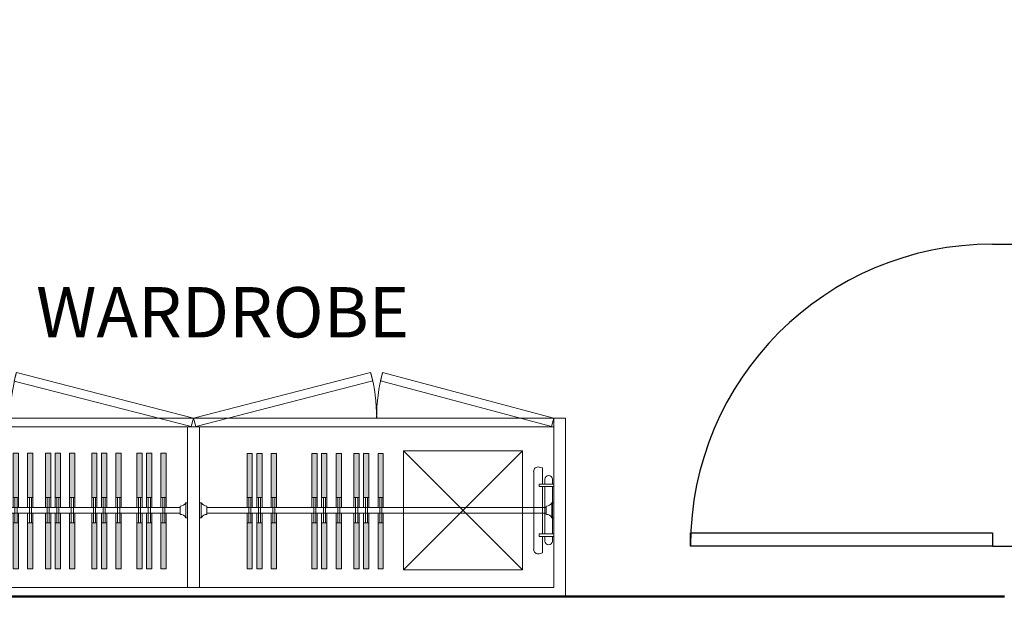
# Model space of a CAD drawing. Units: inches. Extents: x -466983 to 1020, y 324 to 318697.
# Tile 43 of 97: x 491 to 609, y 827 to 898. Entities that reach past the tile are written whole.
import ezdxf

# ---------------------------------------------------------------- set-up
doc = ezdxf.new("R2010")
doc.units = ezdxf.units.IN
doc.header["$MEASUREMENT"] = 0
for name, color, linetype, lineweight in [('A-ANNO-TEXT', 7, 'Continuous', 18), ('A-DOOR', 3, 'Continuous', 25), ('A-FLOR-PATT', 252, 'Continuous', 13), ('A-FURN', 8, 'Continuous', 18), ('A-WALL', 7, 'Continuous', 50)]:
    doc.layers.add(name, color=color, linetype=linetype, lineweight=lineweight)
doc.styles.get("Standard").update_dxf_attribs({"font": 'arial.ttf'})

# ---------------------------------------------------------------- blocks, each defined once
blk = doc.blocks.new('*U33')
for p, q in [((0, 0), (0, -6)), ((40, 0), (40, -6))]:
    blk.add_line(p, q)
blk.add_lwpolyline([(0, 0), (0, 40), (1.75, 40), (1.75, 0)], close=True)
blk.add_arc((0, 0), 40, 0, 90)
blk = doc.blocks.new('Wardrobe')
h = blk.add_hatch(color=256)
h.dxf.hatch_style = 1
h.paths.add_polyline_path([(2766.95, 1539.75), (2766.16, 1539.75), (2766.16, 1532.86), (2766.95, 1532.86)])
h.paths.add_polyline_path([(2766.95, 1529.07), (2766.16, 1529.07), (2766.16, 1522.48), (2766.95, 1522.48)])
h.paths.add_polyline_path([(2799.41, 1529.07), (2798.63, 1529.07), (2798.63, 1522.47), (2799.41, 1522.47)])
h.paths.add_polyline_path([(2799.41, 1539.75), (2798.63, 1539.75), (2798.63, 1532.86), (2799.41, 1532.86)])
h.paths.add_polyline_path([(2813.08, 1539.75), (2812.29, 1539.75), (2812.29, 1532.86), (2813.08, 1532.86)])
h.paths.add_polyline_path([(2813.08, 1529.07), (2812.29, 1529.07), (2812.29, 1522.47), (2813.08, 1522.47)])
h.paths.add_polyline_path([(2825.84, 1539.75), (2825.05, 1539.75), (2825.05, 1532.86), (2825.84, 1532.86)])
h.paths.add_polyline_path([(2825.84, 1529.07), (2825.05, 1529.07), (2825.05, 1522.47), (2825.84, 1522.47)])
h.paths.add_polyline_path([(2782.93, 1539.75), (2782.14, 1539.75), (2782.14, 1532.86), (2782.93, 1532.86)])
h.paths.add_polyline_path([(2782.93, 1529.07), (2782.14, 1529.07), (2782.14, 1522.48), (2782.93, 1522.48)])
h.paths.add_polyline_path([(2838.6, 1539.75), (2837.81, 1539.75), (2837.81, 1532.86), (2838.6, 1532.86)])
h.paths.add_polyline_path([(2838.6, 1529.07), (2837.81, 1529.07), (2837.81, 1522.47), (2838.6, 1522.47)])
h = blk.add_hatch(color=256)
h.dxf.hatch_style = 1
h.paths.add_polyline_path([(2769.11, 1539.75), (2768.32, 1539.75), (2768.32, 1532.86), (2769.11, 1532.86)])
h.paths.add_polyline_path([(2769.11, 1529.07), (2768.32, 1529.07), (2768.32, 1522.48), (2769.11, 1522.48)])
h.paths.add_polyline_path([(2801.57, 1539.75), (2800.79, 1539.75), (2800.79, 1532.86), (2801.57, 1532.86)])
h.paths.add_polyline_path([(2801.57, 1529.07), (2800.79, 1529.07), (2800.79, 1522.47), (2801.57, 1522.47)])
h.paths.add_polyline_path([(2815.24, 1539.75), (2814.45, 1539.75), (2814.45, 1532.86), (2815.24, 1532.86)])
h.paths.add_polyline_path([(2815.24, 1529.07), (2814.45, 1529.07), (2814.45, 1522.47), (2815.24, 1522.47)])
h.paths.add_polyline_path([(2828, 1529.07), (2827.21, 1529.07), (2827.21, 1522.47), (2828, 1522.47)])
h.paths.add_polyline_path([(2828, 1539.75), (2827.21, 1539.75), (2827.21, 1532.86), (2828, 1532.86)])
h.paths.add_polyline_path([(2840.76, 1539.75), (2839.97, 1539.75), (2839.97, 1532.86), (2840.76, 1532.86)])
h.paths.add_polyline_path([(2840.76, 1529.07), (2839.97, 1529.07), (2839.97, 1522.47), (2840.76, 1522.47)])
h.paths.add_polyline_path([(2785.09, 1539.75), (2784.3, 1539.75), (2784.3, 1532.86), (2785.09, 1532.86)])
h.paths.add_polyline_path([(2785.09, 1529.07), (2784.3, 1529.07), (2784.3, 1522.48), (2785.09, 1522.48)])
h = blk.add_hatch(color=256)
h.dxf.hatch_style = 1
h.paths.add_polyline_path([(2770.56, 1539.75), (2769.77, 1539.75), (2769.77, 1532.86), (2770.56, 1532.86)])
h.paths.add_polyline_path([(2770.56, 1529.07), (2769.77, 1529.07), (2769.77, 1522.48), (2770.56, 1522.48)])
h.paths.add_polyline_path([(2786.54, 1539.75), (2785.76, 1539.75), (2785.76, 1532.86), (2786.54, 1532.86)])
h.paths.add_polyline_path([(2786.54, 1529.07), (2785.76, 1529.07), (2785.76, 1522.48), (2786.54, 1522.48)])
h.paths.add_polyline_path([(2803.03, 1539.75), (2802.24, 1539.75), (2802.24, 1532.86), (2803.03, 1532.86)])
h.paths.add_polyline_path([(2803.03, 1529.07), (2802.24, 1529.07), (2802.24, 1522.47), (2803.03, 1522.47)])
h.paths.add_polyline_path([(2816.69, 1539.75), (2815.9, 1539.75), (2815.9, 1532.86), (2816.69, 1532.86)])
h.paths.add_polyline_path([(2816.69, 1529.07), (2815.9, 1529.07), (2815.9, 1522.47), (2816.69, 1522.47)])
h = blk.add_hatch(color=256)
h.dxf.hatch_style = 1
h.paths.add_polyline_path([(2773.22, 1539.75), (2772.43, 1539.75), (2772.43, 1532.86), (2773.22, 1532.86)])
h.paths.add_polyline_path([(2806.16, 1539.75), (2805.37, 1539.75), (2805.37, 1532.86), (2806.16, 1532.86)])
h.paths.add_polyline_path([(2806.16, 1529.07), (2805.37, 1529.07), (2805.37, 1522.47), (2806.16, 1522.47)])
h.paths.add_polyline_path([(2773.22, 1529.07), (2772.43, 1529.07), (2772.43, 1522.48), (2773.22, 1522.48)])
h.paths.add_polyline_path([(2819.35, 1539.75), (2818.56, 1539.75), (2818.56, 1532.86), (2819.35, 1532.86)])
h.paths.add_polyline_path([(2819.35, 1529.07), (2818.56, 1529.07), (2818.56, 1522.47), (2819.35, 1522.47)])
h.paths.add_polyline_path([(2832.33, 1539.75), (2831.54, 1539.75), (2831.54, 1532.86), (2832.33, 1532.86)])
h.paths.add_polyline_path([(2832.33, 1529.07), (2831.54, 1529.07), (2831.54, 1522.47), (2832.33, 1522.47)])
h = blk.add_hatch(color=256)
h.dxf.hatch_style = 1
h.paths.add_polyline_path([(2775.38, 1539.75), (2774.59, 1539.75), (2774.59, 1532.86), (2775.38, 1532.86)])
h.paths.add_polyline_path([(2775.38, 1529.07), (2774.59, 1529.07), (2774.59, 1522.48), (2775.38, 1522.48)])
h.paths.add_polyline_path([(2808.32, 1539.75), (2807.53, 1539.75), (2807.53, 1532.86), (2808.32, 1532.86)])
h.paths.add_polyline_path([(2808.32, 1529.07), (2807.53, 1529.07), (2807.53, 1522.47), (2808.32, 1522.47)])
h.paths.add_polyline_path([(2834.49, 1539.75), (2833.7, 1539.75), (2833.7, 1532.86), (2834.49, 1532.86)])
h.paths.add_polyline_path([(2834.49, 1529.07), (2833.7, 1529.07), (2833.7, 1522.47), (2834.49, 1522.47)])
h = blk.add_hatch(color=256)
h.dxf.hatch_style = 1
h.paths.add_polyline_path([(2776.83, 1539.75), (2776.04, 1539.75), (2776.04, 1532.86), (2776.83, 1532.86)])
h.paths.add_polyline_path([(2776.83, 1529.07), (2776.04, 1529.07), (2776.04, 1522.48), (2776.83, 1522.48)])
h.paths.add_polyline_path([(2809.77, 1539.75), (2808.98, 1539.75), (2808.98, 1532.86), (2809.77, 1532.86)])
h.paths.add_polyline_path([(2809.77, 1529.07), (2808.98, 1529.07), (2808.98, 1522.47), (2809.77, 1522.47)])
h.paths.add_polyline_path([(2821.51, 1539.75), (2820.72, 1539.75), (2820.72, 1532.86), (2821.51, 1532.86)])
h.paths.add_polyline_path([(2821.51, 1529.07), (2820.72, 1529.07), (2820.72, 1522.47), (2821.51, 1522.47)])
h = blk.add_hatch(color=256)
h.dxf.hatch_style = 1
h.paths.add_polyline_path([(2822.96, 1539.75), (2822.17, 1539.75), (2822.17, 1532.86), (2822.96, 1532.86)])
h.paths.add_polyline_path([(2822.96, 1529.07), (2822.17, 1529.07), (2822.17, 1522.47), (2822.96, 1522.47)])
h = blk.add_hatch(color=256)
h.dxf.hatch_style = 1
h.paths.add_polyline_path([(2829.45, 1539.75), (2828.67, 1539.75), (2828.67, 1532.86), (2829.45, 1532.86)])
h.paths.add_polyline_path([(2829.45, 1529.07), (2828.67, 1529.07), (2828.67, 1522.47), (2829.45, 1522.47)])
h.paths.add_polyline_path([(2842.22, 1539.75), (2841.43, 1539.75), (2841.43, 1532.86), (2842.22, 1532.86)])
h.paths.add_polyline_path([(2842.22, 1529.07), (2841.43, 1529.07), (2841.43, 1522.47), (2842.22, 1522.47)])
for p, q in [((2738.89, 1517.19, 0), (2738.89, 1543.9, 0)), ((2738.89, 1543.9, 0), (2850.18, 1543.9, 0)), ((2850.18, 1543.9, 0), (2850.18, 1517.19, 0)), ((2848.4, 1542.57, 0), (2740.67, 1542.57, 0)), ((2740.67, 1542.57, 0), (2740.67, 1517.19, 0)), ((2793.64, 1542.57, 0), (2793.64, 1518.53, 0)), ((2795.43, 1542.57, 0), (2795.43, 1518.53, 0)), ((2848.4, 1517.19, 0), (2848.4, 1542.57, 0)), ((2740.94, 1532.1, 0), (2740.67, 1532.1, 0)), ((2740.94, 1532.1, 0), (2740.67, 1532.1, 0)), ((2740.94, 1532.1, 0), (2740.94, 1529.88, 0)), ((2740.94, 1532.1, 0), (2740.94, 1529.88, 0)), ((2741.78, 1531.61, 0), (2741.78, 1530.37, 0)), ((2741.78, 1531.45, 0), (2792.53, 1531.45, 0)), ((2792.53, 1531.61, 0), (2792.53, 1530.37, 0)), ((2793.38, 1532.1, 0), (2793.38, 1529.88, 0)), ((2793.38, 1532.1, 0), (2793.38, 1529.88, 0)), ((2793.38, 1532.1, 0), (2793.64, 1532.1, 0)), ((2793.38, 1532.1, 0), (2793.64, 1532.1, 0)), ((2795.69, 1532.1, 0), (2795.43, 1532.1, 0)), ((2795.69, 1532.1, 0), (2795.43, 1532.1, 0)), ((2795.69, 1532.1, 0), (2795.69, 1529.88, 0)), ((2795.69, 1532.1, 0), (2795.69, 1529.88, 0)), ((2796.54, 1531.61, 0), (2796.54, 1530.37, 0)), ((2796.54, 1531.45, 0), (2847.29, 1531.45, 0)), ((2847.29, 1531.61, 0), (2847.29, 1530.37, 0)), ((2848.13, 1532.1, 0), (2848.13, 1529.88, 0)), ((2848.13, 1532.1, 0), (2848.13, 1529.88, 0)), ((2848.13, 1532.1, 0), (2848.4, 1532.1, 0)), ((2848.13, 1532.1, 0), (2848.4, 1532.1, 0)), ((2741.78, 1530.56, 0), (2792.53, 1530.56, 0)), ((2796.54, 1530.56, 0), (2847.29, 1530.56, 0)), ((2740.94, 1529.88, 0), (2740.67, 1529.88, 0)), ((2740.94, 1529.88, 0), (2740.67, 1529.88, 0)), ((2793.38, 1529.88, 0), (2793.64, 1529.88, 0)), ((2793.38, 1529.88, 0), (2793.64, 1529.88, 0)), ((2795.69, 1529.88, 0), (2795.43, 1529.88, 0)), ((2795.69, 1529.88, 0), (2795.43, 1529.88, 0)), ((2848.13, 1529.88, 0), (2848.4, 1529.88, 0)), ((2848.13, 1529.88, 0), (2848.4, 1529.88, 0)), ((2848.4, 1518.53, 0), (2740.67, 1518.53, 0)), ((2740.67, 1517.19, 0), (2741.02, 1518.48, 0)), ((2741.02, 1518.48, 0), (2766.6, 1511.65, 0)), ((2794.19, 1518.48, 0), (2767.71, 1511.65, 0)), ((2795.43, 1518.53, 0), (2793.64, 1518.53, 0)), ((2794.53, 1517.19, 0), (2794.19, 1518.48, 0)), ((2794.53, 1517.19, 0), (2794.88, 1518.48, 0)), ((2794.88, 1518.48, 0), (2821.36, 1511.66, 0)), ((2848.05, 1518.48, 0), (2822.47, 1511.66, 0)), ((2848.4, 1517.19, 0), (2848.05, 1518.48, 0)), ((2740.67, 1517.19, 0), (2738.89, 1517.19, 0)), ((2848.4, 1517.19, 0), (2740.67, 1517.19, 0)), ((2766.26, 1510.37, 0), (2740.67, 1517.19, 0)), ((2768.06, 1510.37, 0), (2794.53, 1517.19, 0)), ((2821.01, 1510.37, 0), (2794.53, 1517.19, 0)), ((2822.81, 1510.37, 0), (2848.4, 1517.19, 0)), ((2850.18, 1517.19, 0), (2848.4, 1517.19, 0)), ((2766.6, 1511.65, 0), (2766.26, 1510.37, 0)), ((2767.71, 1511.65, 0), (2768.06, 1510.37, 0)), ((2821.36, 1511.66, 0), (2821.01, 1510.37, 0)), ((2822.47, 1511.66, 0), (2822.81, 1510.37, 0))]:
    blk.add_line(p, q)
at = {"ltscale": 0.106667}
for p, q in [((2745.32, 1522.09, 0), (2763.13, 1539.9, 0)), ((2745.32, 1522.09, 0), (2745.32, 1539.9, 0)), ((2745.32, 1539.9, 0), (2763.13, 1539.9, 0)), ((2763.13, 1522.09, 0), (2745.32, 1539.9, 0)), ((2763.13, 1539.9, 0), (2763.13, 1522.09, 0)), ((2763.13, 1522.09, 0), (2745.32, 1522.09, 0))]:
    blk.add_line(p, q, dxfattribs=at)
at = {"ltscale": 0.037333}
for p, q in [((2766.16, 1531.37, 0), (2766.16, 1539.75, 0)), ((2766.16, 1539.75, 0), (2766.95, 1539.75, 0)), ((2766.95, 1539.75, 0), (2766.95, 1531.37, 0)), ((2768.32, 1531.37, 0), (2768.32, 1539.75, 0)), ((2768.32, 1539.75, 0), (2769.11, 1539.75, 0)), ((2769.11, 1539.75, 0), (2769.11, 1531.37, 0)), ((2769.77, 1531.37, 0), (2769.77, 1539.75, 0)), ((2769.77, 1539.75, 0), (2770.56, 1539.75, 0)), ((2770.56, 1539.75, 0), (2770.56, 1531.37, 0)), ((2772.43, 1531.37, 0), (2772.43, 1539.75, 0)), ((2772.43, 1539.75, 0), (2773.22, 1539.75, 0)), ((2773.22, 1539.75, 0), (2773.22, 1531.37, 0)), ((2774.59, 1531.37, 0), (2774.59, 1539.75, 0)), ((2774.59, 1539.75, 0), (2775.38, 1539.75, 0)), ((2775.38, 1539.75, 0), (2775.38, 1531.37, 0)), ((2776.04, 1531.37, 0), (2776.04, 1539.75, 0)), ((2776.04, 1539.75, 0), (2776.83, 1539.75, 0)), ((2776.83, 1539.75, 0), (2776.83, 1531.37, 0)), ((2782.14, 1531.37, 0), (2782.14, 1539.75, 0)), ((2782.14, 1539.75, 0), (2782.93, 1539.75, 0)), ((2782.93, 1539.75, 0), (2782.93, 1531.37, 0)), ((2784.3, 1531.37, 0), (2784.3, 1539.75, 0)), ((2784.3, 1539.75, 0), (2785.09, 1539.75, 0)), ((2785.09, 1539.75, 0), (2785.09, 1531.37, 0)), ((2785.76, 1531.37, 0), (2785.76, 1539.75, 0)), ((2785.76, 1539.75, 0), (2786.54, 1539.75, 0)), ((2786.54, 1539.75, 0), (2786.54, 1531.37, 0)), ((2798.63, 1531.36, 0), (2798.63, 1539.75, 0)), ((2798.63, 1539.75, 0), (2799.41, 1539.75, 0)), ((2799.41, 1539.75, 0), (2799.41, 1531.36, 0)), ((2800.79, 1531.36, 0), (2800.79, 1539.75, 0)), ((2800.79, 1539.75, 0), (2801.57, 1539.75, 0)), ((2801.57, 1539.75, 0), (2801.57, 1531.36, 0)), ((2802.24, 1531.36, 0), (2802.24, 1539.75, 0)), ((2802.24, 1539.75, 0), (2803.03, 1539.75, 0)), ((2803.03, 1539.75, 0), (2803.03, 1531.36, 0)), ((2805.37, 1531.36, 0), (2805.37, 1539.75, 0)), ((2805.37, 1539.75, 0), (2806.16, 1539.75, 0)), ((2806.16, 1539.75, 0), (2806.16, 1531.36, 0)), ((2807.53, 1531.36, 0), (2807.53, 1539.75, 0)), ((2807.53, 1539.75, 0), (2808.32, 1539.75, 0)), ((2808.32, 1539.75, 0), (2808.32, 1531.36, 0)), ((2808.98, 1531.36, 0), (2808.98, 1539.75, 0)), ((2808.98, 1539.75, 0), (2809.77, 1539.75, 0)), ((2809.77, 1539.75, 0), (2809.77, 1531.36, 0)), ((2812.29, 1531.36, 0), (2812.29, 1539.75, 0)), ((2812.29, 1539.75, 0), (2813.08, 1539.75, 0)), ((2813.08, 1539.75, 0), (2813.08, 1531.36, 0)), ((2814.45, 1531.36, 0), (2814.45, 1539.75, 0)), ((2814.45, 1539.75, 0), (2815.24, 1539.75, 0)), ((2815.24, 1539.75, 0), (2815.24, 1531.36, 0)), ((2815.9, 1531.36, 0), (2815.9, 1539.75, 0)), ((2815.9, 1539.75, 0), (2816.69, 1539.75, 0)), ((2816.69, 1539.75, 0), (2816.69, 1531.36, 0)), ((2818.56, 1531.36, 0), (2818.56, 1539.75, 0)), ((2818.56, 1539.75, 0), (2819.35, 1539.75, 0)), ((2819.35, 1539.75, 0), (2819.35, 1531.36, 0)), ((2820.72, 1531.36, 0), (2820.72, 1539.75, 0)), ((2820.72, 1539.75, 0), (2821.51, 1539.75, 0)), ((2821.51, 1539.75, 0), (2821.51, 1531.36, 0)), ((2822.17, 1531.36, 0), (2822.17, 1539.75, 0)), ((2822.17, 1539.75, 0), (2822.96, 1539.75, 0)), ((2822.96, 1539.75, 0), (2822.96, 1531.36, 0)), ((2825.05, 1531.36, 0), (2825.05, 1539.75, 0)), ((2825.05, 1539.75, 0), (2825.84, 1539.75, 0)), ((2825.84, 1539.75, 0), (2825.84, 1531.36, 0)), ((2827.21, 1531.36, 0), (2827.21, 1539.75, 0)), ((2827.21, 1539.75, 0), (2828, 1539.75, 0)), ((2828, 1539.75, 0), (2828, 1531.36, 0)), ((2828.67, 1531.36, 0), (2828.67, 1539.75, 0)), ((2828.67, 1539.75, 0), (2829.45, 1539.75, 0)), ((2829.45, 1539.75, 0), (2829.45, 1531.36, 0)), ((2831.54, 1531.36, 0), (2831.54, 1539.75, 0)), ((2831.54, 1539.75, 0), (2832.33, 1539.75, 0)), ((2832.33, 1539.75, 0), (2832.33, 1531.36, 0)), ((2833.7, 1531.36, 0), (2833.7, 1539.75, 0)), ((2833.7, 1539.75, 0), (2834.49, 1539.75, 0)), ((2834.49, 1539.75, 0), (2834.49, 1531.36, 0)), ((2835.16, 1531.36, 0), (2835.16, 1539.75, 0)), ((2835.16, 1539.75, 0), (2835.95, 1539.75, 0)), ((2835.95, 1539.75, 0), (2835.95, 1531.36, 0)), ((2837.81, 1531.36, 0), (2837.81, 1539.75, 0)), ((2837.81, 1539.75, 0), (2838.6, 1539.75, 0)), ((2838.6, 1539.75, 0), (2838.6, 1531.36, 0)), ((2839.97, 1531.36, 0), (2839.97, 1539.75, 0)), ((2839.97, 1539.75, 0), (2840.76, 1539.75, 0)), ((2840.76, 1539.75, 0), (2840.76, 1531.36, 0)), ((2841.43, 1531.36, 0), (2841.43, 1539.75, 0)), ((2841.43, 1539.75, 0), (2842.22, 1539.75, 0)), ((2842.22, 1539.75, 0), (2842.22, 1531.36, 0)), ((2766.16, 1532.86, 0), (2766.95, 1532.86, 0)), ((2766.37, 1529.07, 0), (2766.37, 1532.86, 0)), ((2766.69, 1529.07, 0), (2766.69, 1532.86, 0)), ((2768.32, 1532.86, 0), (2769.11, 1532.86, 0)), ((2768.53, 1529.07, 0), (2768.53, 1532.86, 0)), ((2768.84, 1529.07, 0), (2768.84, 1532.86, 0)), ((2769.77, 1532.86, 0), (2770.56, 1532.86, 0)), ((2769.99, 1529.07, 0), (2769.99, 1532.86, 0)), ((2770.3, 1529.07, 0), (2770.3, 1532.86, 0)), ((2772.43, 1532.86, 0), (2773.22, 1532.86, 0)), ((2772.64, 1529.07, 0), (2772.64, 1532.86, 0)), ((2772.96, 1529.07, 0), (2772.96, 1532.86, 0)), ((2774.59, 1532.86, 0), (2775.38, 1532.86, 0)), ((2774.8, 1529.07, 0), (2774.8, 1532.86, 0)), ((2775.11, 1529.07, 0), (2775.11, 1532.86, 0)), ((2776.04, 1532.86, 0), (2776.83, 1532.86, 0)), ((2776.26, 1529.07, 0), (2776.26, 1532.86, 0)), ((2776.57, 1529.07, 0), (2776.57, 1532.86, 0)), ((2782.14, 1532.86, 0), (2782.93, 1532.86, 0)), ((2782.36, 1529.07, 0), (2782.36, 1532.86, 0)), ((2782.67, 1529.07, 0), (2782.67, 1532.86, 0)), ((2784.3, 1532.86, 0), (2785.09, 1532.86, 0)), ((2784.52, 1529.07, 0), (2784.52, 1532.86, 0)), ((2784.83, 1529.07, 0), (2784.83, 1532.86, 0)), ((2785.76, 1532.86, 0), (2786.54, 1532.86, 0)), ((2785.97, 1529.07, 0), (2785.97, 1532.86, 0)), ((2786.28, 1529.07, 0), (2786.28, 1532.86, 0)), ((2798.63, 1532.86, 0), (2799.41, 1532.86, 0)), ((2798.84, 1529.07, 0), (2798.84, 1532.86, 0)), ((2799.15, 1529.07, 0), (2799.15, 1532.86, 0)), ((2800.79, 1532.86, 0), (2801.57, 1532.86, 0)), ((2801, 1529.07, 0), (2801, 1532.86, 0)), ((2801.31, 1529.07, 0), (2801.31, 1532.86, 0)), ((2802.24, 1532.86, 0), (2803.03, 1532.86, 0)), ((2802.45, 1529.07, 0), (2802.45, 1532.86, 0)), ((2802.76, 1529.07, 0), (2802.76, 1532.86, 0)), ((2805.37, 1532.86, 0), (2806.16, 1532.86, 0)), ((2805.58, 1529.07, 0), (2805.58, 1532.86, 0)), ((2805.9, 1529.07, 0), (2805.9, 1532.86, 0)), ((2807.53, 1532.86, 0), (2808.32, 1532.86, 0)), ((2807.74, 1529.07, 0), (2807.74, 1532.86, 0)), ((2808.06, 1529.07, 0), (2808.06, 1532.86, 0)), ((2808.98, 1532.86, 0), (2809.77, 1532.86, 0)), ((2809.2, 1529.07, 0), (2809.2, 1532.86, 0)), ((2809.51, 1529.07, 0), (2809.51, 1532.86, 0)), ((2812.29, 1532.86, 0), (2813.08, 1532.86, 0)), ((2812.51, 1529.07, 0), (2812.51, 1532.86, 0)), ((2812.82, 1529.07, 0), (2812.82, 1532.86, 0)), ((2814.45, 1532.86, 0), (2815.24, 1532.86, 0)), ((2814.67, 1529.07, 0), (2814.67, 1532.86, 0)), ((2814.98, 1529.07, 0), (2814.98, 1532.86, 0)), ((2815.9, 1532.86, 0), (2816.69, 1532.86, 0)), ((2816.12, 1529.07, 0), (2816.12, 1532.86, 0)), ((2816.43, 1529.07, 0), (2816.43, 1532.86, 0)), ((2818.56, 1532.86, 0), (2819.35, 1532.86, 0)), ((2818.78, 1529.07, 0), (2818.78, 1532.86, 0)), ((2819.09, 1529.07, 0), (2819.09, 1532.86, 0)), ((2820.72, 1532.86, 0), (2821.51, 1532.86, 0)), ((2820.94, 1529.07, 0), (2820.94, 1532.86, 0)), ((2821.25, 1529.07, 0), (2821.25, 1532.86, 0)), ((2822.17, 1532.86, 0), (2822.96, 1532.86, 0)), ((2822.39, 1529.07, 0), (2822.39, 1532.86, 0)), ((2822.7, 1529.07, 0), (2822.7, 1532.86, 0)), ((2825.05, 1532.86, 0), (2825.84, 1532.86, 0)), ((2825.27, 1529.07, 0), (2825.27, 1532.86, 0)), ((2825.58, 1529.07, 0), (2825.58, 1532.86, 0)), ((2827.21, 1532.86, 0), (2828, 1532.86, 0)), ((2827.43, 1529.07, 0), (2827.43, 1532.86, 0)), ((2827.74, 1529.07, 0), (2827.74, 1532.86, 0)), ((2828.67, 1532.86, 0), (2829.45, 1532.86, 0)), ((2828.88, 1529.07, 0), (2828.88, 1532.86, 0)), ((2829.19, 1529.07, 0), (2829.19, 1532.86, 0)), ((2831.54, 1532.86, 0), (2832.33, 1532.86, 0)), ((2831.76, 1529.07, 0), (2831.76, 1532.86, 0)), ((2832.07, 1529.07, 0), (2832.07, 1532.86, 0)), ((2833.7, 1532.86, 0), (2834.49, 1532.86, 0)), ((2833.92, 1529.07, 0), (2833.92, 1532.86, 0)), ((2834.23, 1529.07, 0), (2834.23, 1532.86, 0)), ((2835.16, 1532.86, 0), (2835.95, 1532.86, 0)), ((2835.37, 1529.07, 0), (2835.37, 1532.86, 0)), ((2835.68, 1529.07, 0), (2835.68, 1532.86, 0)), ((2837.81, 1532.86, 0), (2838.6, 1532.86, 0)), ((2838.03, 1529.07, 0), (2838.03, 1532.86, 0)), ((2838.34, 1529.07, 0), (2838.34, 1532.86, 0)), ((2839.97, 1532.86, 0), (2840.76, 1532.86, 0)), ((2840.19, 1529.07, 0), (2840.19, 1532.86, 0)), ((2840.5, 1529.07, 0), (2840.5, 1532.86, 0)), ((2841.43, 1532.86, 0), (2842.22, 1532.86, 0)), ((2841.64, 1529.07, 0), (2841.64, 1532.86, 0)), ((2841.95, 1529.07, 0), (2841.95, 1532.86, 0)), ((2766.16, 1522.48, 0), (2766.16, 1530.56, 0)), ((2766.95, 1530.56, 0), (2766.95, 1522.48, 0)), ((2768.32, 1522.48, 0), (2768.32, 1530.56, 0)), ((2769.11, 1530.56, 0), (2769.11, 1522.48, 0)), ((2769.77, 1522.48, 0), (2769.77, 1530.56, 0)), ((2770.56, 1530.56, 0), (2770.56, 1522.48, 0)), ((2772.43, 1522.48, 0), (2772.43, 1530.56, 0)), ((2773.22, 1530.56, 0), (2773.22, 1522.48, 0)), ((2774.59, 1522.48, 0), (2774.59, 1530.56, 0)), ((2775.38, 1530.56, 0), (2775.38, 1522.48, 0)), ((2776.04, 1522.48, 0), (2776.04, 1530.56, 0)), ((2776.83, 1530.56, 0), (2776.83, 1522.48, 0)), ((2782.14, 1522.48, 0), (2782.14, 1530.56, 0)), ((2782.93, 1530.56, 0), (2782.93, 1522.48, 0)), ((2784.3, 1522.48, 0), (2784.3, 1530.56, 0)), ((2785.09, 1530.56, 0), (2785.09, 1522.48, 0)), ((2785.76, 1522.48, 0), (2785.76, 1530.56, 0)), ((2786.54, 1530.56, 0), (2786.54, 1522.48, 0)), ((2798.63, 1522.47, 0), (2798.63, 1530.56, 0)), ((2799.41, 1530.56, 0), (2799.41, 1522.47, 0)), ((2800.79, 1522.47, 0), (2800.79, 1530.56, 0)), ((2801.57, 1530.56, 0), (2801.57, 1522.47, 0)), ((2802.24, 1522.47, 0), (2802.24, 1530.56, 0)), ((2803.03, 1530.56, 0), (2803.03, 1522.47, 0)), ((2805.37, 1522.47, 0), (2805.37, 1530.56, 0)), ((2806.16, 1530.56, 0), (2806.16, 1522.47, 0)), ((2807.53, 1522.47, 0), (2807.53, 1530.56, 0)), ((2808.32, 1530.56, 0), (2808.32, 1522.47, 0)), ((2808.98, 1522.47, 0), (2808.98, 1530.56, 0)), ((2809.77, 1530.56, 0), (2809.77, 1522.47, 0)), ((2812.29, 1522.47, 0), (2812.29, 1530.56, 0)), ((2813.08, 1530.56, 0), (2813.08, 1522.47, 0)), ((2814.45, 1522.47, 0), (2814.45, 1530.56, 0)), ((2815.24, 1530.56, 0), (2815.24, 1522.47, 0)), ((2815.9, 1522.47, 0), (2815.9, 1530.56, 0)), ((2816.69, 1530.56, 0), (2816.69, 1522.47, 0)), ((2818.56, 1522.47, 0), (2818.56, 1530.56, 0)), ((2819.35, 1530.56, 0), (2819.35, 1522.47, 0)), ((2820.72, 1522.47, 0), (2820.72, 1530.56, 0)), ((2821.51, 1530.56, 0), (2821.51, 1522.47, 0)), ((2822.17, 1522.47, 0), (2822.17, 1530.56, 0)), ((2822.96, 1530.56, 0), (2822.96, 1522.47, 0)), ((2825.05, 1522.47, 0), (2825.05, 1530.56, 0)), ((2825.84, 1530.56, 0), (2825.84, 1522.47, 0)), ((2827.21, 1522.47, 0), (2827.21, 1530.56, 0)), ((2828, 1530.56, 0), (2828, 1522.47, 0)), ((2828.67, 1522.47, 0), (2828.67, 1530.56, 0)), ((2829.45, 1530.56, 0), (2829.45, 1522.47, 0)), ((2831.54, 1522.47, 0), (2831.54, 1530.56, 0)), ((2832.33, 1530.56, 0), (2832.33, 1522.47, 0)), ((2833.7, 1522.47, 0), (2833.7, 1530.56, 0)), ((2834.49, 1530.56, 0), (2834.49, 1522.47, 0)), ((2835.16, 1522.47, 0), (2835.16, 1530.56, 0)), ((2835.95, 1530.56, 0), (2835.95, 1522.47, 0)), ((2837.81, 1522.47, 0), (2837.81, 1530.56, 0)), ((2838.6, 1530.56, 0), (2838.6, 1522.47, 0)), ((2839.97, 1522.47, 0), (2839.97, 1530.56, 0)), ((2840.76, 1530.56, 0), (2840.76, 1522.47, 0)), ((2841.43, 1522.47, 0), (2841.43, 1530.56, 0)), ((2842.22, 1530.56, 0), (2842.22, 1522.47, 0)), ((2766.16, 1529.07, 0), (2766.95, 1529.07, 0)), ((2768.32, 1529.07, 0), (2769.11, 1529.07, 0)), ((2769.77, 1529.07, 0), (2770.56, 1529.07, 0)), ((2772.43, 1529.07, 0), (2773.22, 1529.07, 0)), ((2774.59, 1529.07, 0), (2775.38, 1529.07, 0)), ((2776.04, 1529.07, 0), (2776.83, 1529.07, 0)), ((2782.14, 1529.07, 0), (2782.93, 1529.07, 0)), ((2784.3, 1529.07, 0), (2785.09, 1529.07, 0)), ((2785.76, 1529.07, 0), (2786.54, 1529.07, 0)), ((2798.63, 1529.07, 0), (2799.41, 1529.07, 0)), ((2800.79, 1529.07, 0), (2801.57, 1529.07, 0)), ((2802.24, 1529.07, 0), (2803.03, 1529.07, 0)), ((2805.37, 1529.07, 0), (2806.16, 1529.07, 0)), ((2807.53, 1529.07, 0), (2808.32, 1529.07, 0)), ((2808.98, 1529.07, 0), (2809.77, 1529.07, 0)), ((2812.29, 1529.07, 0), (2813.08, 1529.07, 0)), ((2814.45, 1529.07, 0), (2815.24, 1529.07, 0)), ((2815.9, 1529.07, 0), (2816.69, 1529.07, 0)), ((2818.56, 1529.07, 0), (2819.35, 1529.07, 0)), ((2820.72, 1529.07, 0), (2821.51, 1529.07, 0)), ((2822.17, 1529.07, 0), (2822.96, 1529.07, 0)), ((2825.05, 1529.07, 0), (2825.84, 1529.07, 0)), ((2827.21, 1529.07, 0), (2828, 1529.07, 0)), ((2828.67, 1529.07, 0), (2829.45, 1529.07, 0)), ((2831.54, 1529.07, 0), (2832.33, 1529.07, 0)), ((2833.7, 1529.07, 0), (2834.49, 1529.07, 0)), ((2835.16, 1529.07, 0), (2835.95, 1529.07, 0)), ((2837.81, 1529.07, 0), (2838.6, 1529.07, 0)), ((2839.97, 1529.07, 0), (2840.76, 1529.07, 0)), ((2841.43, 1529.07, 0), (2842.22, 1529.07, 0)), ((2766.95, 1522.48, 0), (2766.16, 1522.48, 0)), ((2769.11, 1522.48, 0), (2768.32, 1522.48, 0)), ((2770.56, 1522.48, 0), (2769.77, 1522.48, 0)), ((2773.22, 1522.48, 0), (2772.43, 1522.48, 0)), ((2775.38, 1522.48, 0), (2774.59, 1522.48, 0)), ((2776.83, 1522.48, 0), (2776.04, 1522.48, 0)), ((2782.93, 1522.48, 0), (2782.14, 1522.48, 0)), ((2785.09, 1522.48, 0), (2784.3, 1522.48, 0)), ((2786.54, 1522.48, 0), (2785.76, 1522.48, 0)), ((2799.41, 1522.47, 0), (2798.63, 1522.47, 0)), ((2801.57, 1522.47, 0), (2800.79, 1522.47, 0)), ((2803.03, 1522.47, 0), (2802.24, 1522.47, 0)), ((2806.16, 1522.47, 0), (2805.37, 1522.47, 0)), ((2808.32, 1522.47, 0), (2807.53, 1522.47, 0)), ((2809.77, 1522.47, 0), (2808.98, 1522.47, 0)), ((2813.08, 1522.47, 0), (2812.29, 1522.47, 0)), ((2815.24, 1522.47, 0), (2814.45, 1522.47, 0)), ((2816.69, 1522.47, 0), (2815.9, 1522.47, 0)), ((2819.35, 1522.47, 0), (2818.56, 1522.47, 0)), ((2821.51, 1522.47, 0), (2820.72, 1522.47, 0)), ((2822.96, 1522.47, 0), (2822.17, 1522.47, 0)), ((2825.84, 1522.47, 0), (2825.05, 1522.47, 0)), ((2828, 1522.47, 0), (2827.21, 1522.47, 0)), ((2829.45, 1522.47, 0), (2828.67, 1522.47, 0)), ((2832.33, 1522.47, 0), (2831.54, 1522.47, 0)), ((2834.49, 1522.47, 0), (2833.7, 1522.47, 0)), ((2835.95, 1522.47, 0), (2835.16, 1522.47, 0)), ((2838.6, 1522.47, 0), (2837.81, 1522.47, 0)), ((2840.76, 1522.47, 0), (2839.97, 1522.47, 0)), ((2842.22, 1522.47, 0), (2841.43, 1522.47, 0))]:
    blk.add_line(p, q, dxfattribs=at)
at = {"ltscale": 0.02}
for p, q in [((2742.34, 1537.37, 0), (2742.84, 1537.5, 0)), ((2742.34, 1534.92, 0), (2742.34, 1537.37, 0)), ((2743.67, 1536.85, 0), (2743.67, 1525.18, 0)), ((2740.67, 1534.92, 0), (2742.84, 1534.92, 0)), ((2742.84, 1534.53, 0), (2740.67, 1534.53, 0)), ((2740.87, 1534.92, 0), (2740.87, 1535.62, 0)), ((2740.87, 1527.45, 0), (2740.87, 1534.53, 0)), ((2741.99, 1535.62, 0), (2741.99, 1534.92, 0)), ((2741.99, 1534.53, 0), (2741.99, 1527.45, 0)), ((2742.34, 1527.45, 0), (2742.34, 1534.53, 0)), ((2742.84, 1534.92, 0), (2742.84, 1534.53, 0)), ((2742.84, 1527.45, 0), (2740.67, 1527.45, 0)), ((2740.67, 1527.07, 0), (2742.84, 1527.07, 0)), ((2740.87, 1526.34, 0), (2740.87, 1527.07, 0)), ((2741.99, 1527.07, 0), (2741.99, 1526.34, 0)), ((2742.34, 1524.65, 0), (2742.34, 1527.07, 0)), ((2742.84, 1527.07, 0), (2742.84, 1527.45, 0)), ((2742.86, 1524.53, 0), (2742.34, 1524.65, 0))]:
    blk.add_line(p, q, dxfattribs=at)
for centre, radius, start, end in [((2743.01, 1536.85, 0), 0.668, 360, 104.1887), ((2741.43, 1535.62, 0), 0.556, 0, 180), ((2741.43, 1526.34, 0), 0.556, 180, 0), ((2743.01, 1525.18, 0), 0.668, 257.5257, 0)]:
    blk.add_arc(centre, radius, start, end, dxfattribs=at)
for centre, radius, start, end in [((2741.78, 1532.59, 0), 0.977, 209.9156, 269.9473), ((2741.78, 1532.59, 0), 0.977, 209.9156, 269.9473), ((2792.53, 1532.59, 0), 0.977, 270.0527, 330.0844), ((2792.53, 1532.59, 0), 0.977, 270.0527, 330.0844), ((2796.54, 1532.59, 0), 0.977, 209.9156, 269.9473), ((2796.54, 1532.59, 0), 0.977, 209.9156, 269.9473), ((2847.29, 1532.59, 0), 0.977, 270.0527, 330.0844), ((2847.29, 1532.59, 0), 0.977, 270.0527, 330.0844), ((2741.78, 1529.39, 0), 0.977, 90.0527, 150.0844), ((2792.53, 1529.39, 0), 0.977, 29.9156, 89.9473), ((2796.54, 1529.39, 0), 0.977, 90.0527, 150.0844), ((2847.29, 1529.39, 0), 0.977, 29.9156, 89.9473), ((2740.78, 1517.19, 0), 26.38, 345.1891, 0), ((2793.53, 1517.19, 0), 26.38, 180, 194.8109), ((2795.54, 1517.19, 0), 26.38, 345.1891, 0), ((2848.29, 1517.19, 0), 26.38, 180, 194.8109)]:
    blk.add_arc(centre, radius, start, end)

msp = doc.modelspace()

# ---------------------------------------------------------------- hatches: boundary and pattern name
at = {"layer": 'A-FLOR-PATT', "transparency": 33554572}
h = msp.add_hatch(dxfattribs=at)
h.set_pattern_fill('ANSI37', color=256, scale=30)
h.set_pattern_definition([(45, (-1212.4137, -290.035), (-2.6516504, 2.6516504), []), (135, (-1212.4137, -290.035), (-2.6516504, -2.6516504), [])])
h.paths.add_polyline_path([(901.81, 1075.94), (900.61, 1075.94), (900.61, 1065.39), (899.39, 1065.39), (898.09, 1065.39), (892.84, 1058.71, -0.258377), (892.19, 1058.35), (879.98, 1058.35, -0.20177), (879.44, 1058.58), (874.08, 1065.39), (872.78, 1065.39), (871.56, 1065.39), (871.56, 1075.94), (813.81, 1075.94), (813.81, 1044.79), (832.39, 1044.79, -0.394795), (848.66, 1028.54), (848.66, 1009.94), (901.81, 1009.94), (901.81, 1015.94), (901.31, 1015.94), (871.31, 1015.94), (871.31, 1017.25), (871.33, 1017.25, -0.401453), (901.31, 1045.94), (901.81, 1045.94)])
edge = h.paths.add_edge_path(flags=16)
edge.add_line((847.77, 1068.95), (847.77, 1073.71))
edge.add_arc((849.23, 1073.71), 1.45, 90, 180, ccw=False)
edge.add_line((849.23, 1075.16), (864.49, 1075.16))
edge.add_arc((864.49, 1073.71), 1.45, 0, 90, ccw=False)
edge.add_line((865.95, 1073.71), (865.95, 1069))
edge.add_arc((832.64, 1068.98), 33.3, -20.6123, 0.0472, ccw=False)
edge.add_ellipse((856.86, 1058.48), major_axis=(0, 10.21), ratio=0.685919, start_angle=100.0088, end_angle=259.9912, ccw=False)
edge.add_arc((881.07, 1068.98), 33.3, 180.0472, 200.6123, ccw=False)
h.paths.add_polyline_path([(853.15, 1066.48), (853.15, 1066.45), (853.15, 1066.45, 0.433107), (852.92, 1066.68), (852.92, 1066.45), (853.15, 1066.45), (853.15, 1066.48), (853.09, 1066.61, 0.697939), (852.7, 1066.45), (852.7, 1066.45), (852.7, 1066.48), (852.92, 1067), (852.92, 1066.68, -0.396254)], flags=0)
h.paths.add_polyline_path([(861.02, 1066.48), (861.02, 1066.45), (861.02, 1066.45, 0.416404), (860.8, 1066.68), (860.8, 1066.45), (861.02, 1066.45), (861.02, 1066.48), (860.97, 1066.61, 0.713344), (860.57, 1066.45), (860.57, 1066.45), (860.57, 1066.48), (860.8, 1067), (860.8, 1066.68, -0.379973)], flags=0)
edge = h.paths.add_edge_path(flags=0)
edge.add_spline(control_points=[(861.13, 1065.79), (861.47, 1065.25), (861.61, 1065.02), (861.98, 1064.37), (862.19, 1063.94), (862.56, 1063.04), (862.72, 1062.56), (862.99, 1061.58), (863.09, 1061.07), (863.25, 1060.03), (863.29, 1059.5), (863.33, 1058.44), (863.32, 1057.91), (863.24, 1056.85), (863.17, 1056.33), (862.97, 1055.31), (862.84, 1054.81), (862.54, 1053.85), (862.36, 1053.39), (861.95, 1052.52), (861.73, 1052.12), (861.23, 1051.36), (860.97, 1051.02), (860.4, 1050.39), (860.11, 1050.12), (859.49, 1049.65), (859.18, 1049.45), (858.53, 1049.13), (858.2, 1049.01), (857.53, 1048.85), (857.2, 1048.81), (856.52, 1048.81), (856.19, 1048.85), (855.52, 1049.01), (855.19, 1049.13), (854.54, 1049.45), (854.23, 1049.64), (853.61, 1050.12), (853.32, 1050.39), (852.75, 1051.01), (852.49, 1051.36), (852, 1052.11), (851.77, 1052.52), (851.36, 1053.39), (851.18, 1053.85), (850.88, 1054.81), (850.75, 1055.31), (850.55, 1056.33), (850.48, 1056.85), (850.4, 1057.9), (850.39, 1058.44), (850.43, 1059.5), (850.47, 1060.03), (850.63, 1061.07), (850.73, 1061.58), (851, 1062.56), (851.16, 1063.04), (851.53, 1063.94), (851.73, 1064.37), (852.11, 1065.02), (852.25, 1065.25), (852.61, 1065.73)], knot_values=[3.915332, 3.915332, 3.915332, 3.915332, 4.013468, 4.013468, 4.175532, 4.175532, 4.337596, 4.337596, 4.49966, 4.49966, 4.661724, 4.661724, 4.823788, 4.823788, 4.985852, 4.985852, 5.147916, 5.147916, 5.30998, 5.30998, 5.472044, 5.472044, 5.634109, 5.634109, 5.796173, 5.796173, 5.958237, 5.958237, 6.120301, 6.120301, 6.282365, 6.282365, 6.444429, 6.444429, 6.606493, 6.606493, 6.768557, 6.768557, 6.930621, 6.930621, 7.092685, 7.092685, 7.254749, 7.254749, 7.416813, 7.416813, 7.578878, 7.578878, 7.740942, 7.740942, 7.903006, 7.903006, 8.06507, 8.06507, 8.227134, 8.227134, 8.389198, 8.389198, 8.551262, 8.551262, 8.65037, 8.65037, 8.65037, 8.65037], degree=3, periodic=0)
edge.add_line((852.64, 1065.79), (861.13, 1065.79))
edge = h.paths.add_edge_path(flags=0)
edge.add_ellipse((856.85, 1057.74), major_axis=(0, 7.79), ratio=0.687861, start_angle=0, end_angle=360)
h.paths.add_polyline_path([(848.86, 1069.39), (848.86, 1073.96, -0.414214), (849.95, 1075.05), (863.77, 1075.05, -0.414214), (864.86, 1073.96), (864.86, 1069.39, -0.388936), (864.52, 1069.03, -0.043561), (849.2, 1069.03, -0.388936)], flags=0)
h.paths.add_polyline_path([(853.1, 1068.11, -1), (852.68, 1068.11, -1)], flags=0)
edge = h.paths.add_edge_path(flags=0)
edge.add_ellipse((856.86, 1057.34), major_axis=(0, 2.21), ratio=0.657164, start_angle=0, end_angle=360)
h.paths.add_polyline_path([(861.04, 1068.11, -1), (860.62, 1068.11, -1)], flags=0)
edge = h.paths.add_edge_path()
edge.add_line((573.95, 1057.34), (573.95, 1075.94))
edge.add_line((573.95, 1075.94), (558.73, 1075.94))
edge.add_line((558.73, 1075.94), (558.73, 1065.39))
edge.add_line((558.73, 1065.39), (557.51, 1065.39))
edge.add_line((557.51, 1065.39), (556.21, 1065.39))
edge.add_line((556.21, 1065.39), (550.95, 1058.71))
edge.add_arc((550.3, 1059.12), 0.765, 270, 327.9483, ccw=False)
edge.add_line((550.3, 1058.35), (538.1, 1058.35))
edge.add_arc((538.1, 1059.12), 0.765, 224.3704, 270, ccw=False)
edge.add_line((537.55, 1058.58), (532.2, 1065.39))
edge.add_line((532.2, 1065.39), (530.9, 1065.39))
edge.add_line((530.9, 1065.39), (529.67, 1065.39))
edge.add_line((529.67, 1065.39), (529.67, 1075.94))
edge.add_line((529.67, 1075.94), (520.81, 1075.94))
edge.add_line((520.81, 1075.94), (520.81, 1045.94))
edge.add_line((520.81, 1045.94), (521.31, 1045.94))
edge.add_arc((521.31, 1015.94), 30, 2.5075, 90, ccw=False)
edge.add_line((551.28, 1017.25), (551.31, 1017.25))
edge.add_line((551.31, 1017.25), (551.31, 1015.94))
edge.add_line((551.31, 1015.94), (520.81, 1015.94))
edge.add_line((520.81, 1015.94), (520.81, 1009.94))
edge.add_line((520.81, 1009.94), (559.19, 1010.4))
edge.add_arc((559.19, 1011.86), 1.45, 180, 270, ccw=False)
edge.add_line((557.74, 1011.86), (557.74, 1016.56))
edge.add_arc((591.04, 1016.59), 33.3, 159.3877, 180.0472, ccw=False)
edge.add_ellipse((566.82, 1027.08), major_axis=(0, 10.21), ratio=0.685919, start_angle=280.0088, end_angle=439.9912, ccw=False)
edge.add_arc((542.61, 1016.59), 33.3, 0.0472, 20.6123, ccw=False)
edge.add_line((575.91, 1016.62), (575.91, 1011.86))
edge.add_arc((574.46, 1011.86), 1.45, -90, 0, ccw=False)
edge.add_line((574.46, 1010.4), (608.81, 1009.94))
edge.add_line((608.81, 1009.94), (608.81, 1041.09))
edge.add_line((608.81, 1041.09), (590.22, 1041.09))
edge.add_arc((590.78, 1057.91), 16.83, 181.9277, 268.1032, ccw=False)
edge = h.paths.add_edge_path()
edge.add_ellipse((494.24, 583.62), major_axis=(0, 10.21), ratio=0.685919, start_angle=280.0088, end_angle=439.9912, ccw=False)
edge.add_arc((470.03, 573.12), 33.3, 0.0472, 20.6123, ccw=False)
edge.add_line((503.33, 573.15), (503.33, 568.39))
edge.add_arc((501.88, 568.39), 1.45, -90, 0, ccw=False)
edge.add_line((501.88, 566.94), (539.81, 566.94))
edge.add_line((539.81, 566.94), (539.81, 572.94))
edge.add_line((539.81, 572.94), (539.31, 572.94))
edge.add_line((539.31, 572.94), (509.31, 572.94))
edge.add_line((509.31, 572.94), (509.31, 574.25))
edge.add_line((509.31, 574.25), (509.33, 574.25))
edge.add_arc((539.31, 572.94), 30, 90, 177.4925, ccw=False)
edge.add_line((539.31, 602.94), (539.81, 602.94))
edge.add_line((539.81, 602.94), (539.81, 626.94))
edge.add_line((539.81, 626.94), (531.77, 626.94))
edge.add_line((531.77, 626.94), (531.77, 616.39))
edge.add_line((531.77, 616.39), (530.55, 616.39))
edge.add_line((530.55, 616.39), (529.25, 616.39))
edge.add_line((529.25, 616.39), (523.71, 609.35))
edge.add_line((523.71, 609.35), (510.78, 609.35))
edge.add_line((510.78, 609.35), (505.24, 616.39))
edge.add_line((505.24, 616.39), (503.94, 616.39))
edge.add_line((503.94, 616.39), (502.72, 616.39))
edge.add_line((502.72, 616.39), (502.72, 626.94))
edge.add_line((502.72, 626.94), (481.7, 626.94))
edge.add_line((481.7, 626.94), (481.7, 611))
edge.add_arc((467.27, 611.47), 14.44, 271.9277, 358.1032, ccw=False)
edge.add_line((467.76, 597.05), (451.81, 597.05))
edge.add_line((451.81, 597.05), (451.81, 584.4))
edge.add_line((451.81, 584.4), (451.81, 566.94))
edge.add_line((451.81, 566.94), (486.61, 566.94))
edge.add_arc((486.61, 568.39), 1.45, 180, 270, ccw=False)
edge.add_line((485.16, 568.39), (485.16, 573.1))
edge.add_arc((518.46, 573.12), 33.3, 159.3877, 180.0472, ccw=False)
h.paths.add_polyline_path([(836.26, 1020.73), (879.89, 1020.73), (879.89, 1039.39), (836.26, 1039.39)], flags=25)
h.paths.add_polyline_path([(549.99, 1036.75), (593.61, 1036.75), (593.61, 1055.41), (549.99, 1055.41)], flags=24)
h.paths.add_polyline_path([(475.12, 595.6), (518.75, 595.6), (518.75, 614.25), (475.12, 614.25)], flags=24)

# ---------------------------------------------------------------- linework, layer by layer
at = {"layer": 'A-WALL'}
msp.add_line((608.81, 828.94), (451.81, 828.94), dxfattribs=at)

# ---------------------------------------------------------------- block references
at = {"layer": 'A-DOOR', "xscale": 0.9000000000000004, "yscale": 0.9000000000000004, "zscale": 0.9000000000000004, "rotation": 90}
msp.add_blockref('*U33', (607.41, 834.94), dxfattribs=at)
at = {"layer": 'A-FURN', "xscale": 0.7967580954171016, "yscale": 0.7967580954171016, "zscale": 0.7967580954171016, "rotation": 180}
msp.add_blockref('Wardrobe', (2738.77, 2059.05), dxfattribs=at)

# ---------------------------------------------------------------- texts
at = {"layer": 'A-ANNO-TEXT', "insert": (400.89, 865.82), "char_height": 6, "attachment_point": 1}
msp.add_mtext_dynamic_manual_height_columns('\\pxqc;WARDROBE', width=229.5583, gutter_width=1, heights=[0], dxfattribs=at)

doc.saveas('drawing.dxf')
